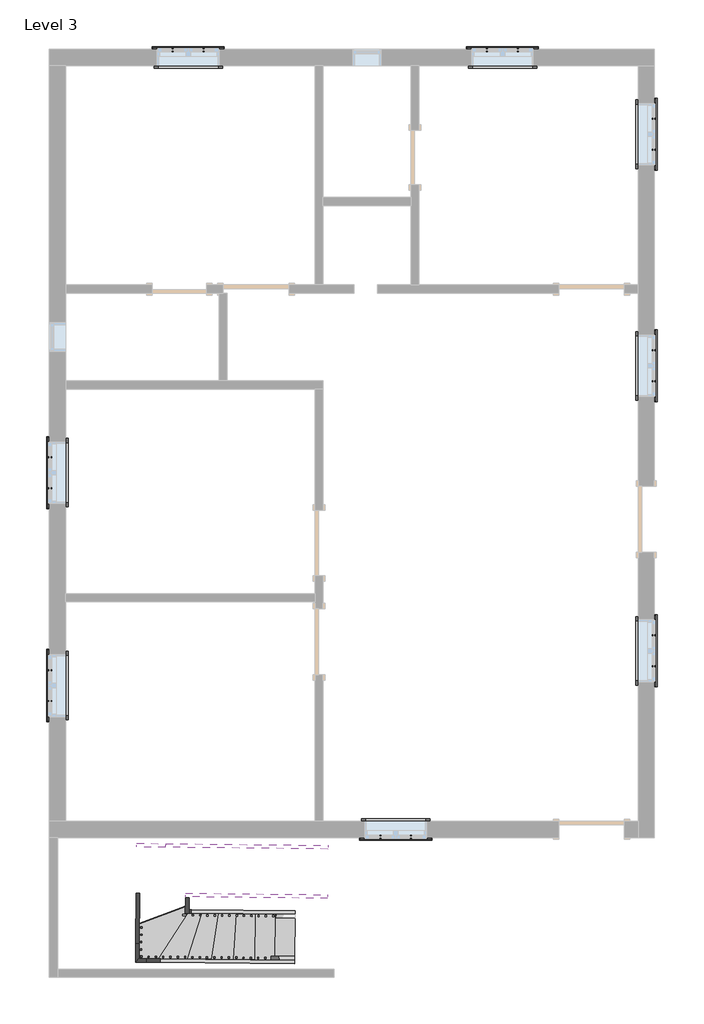
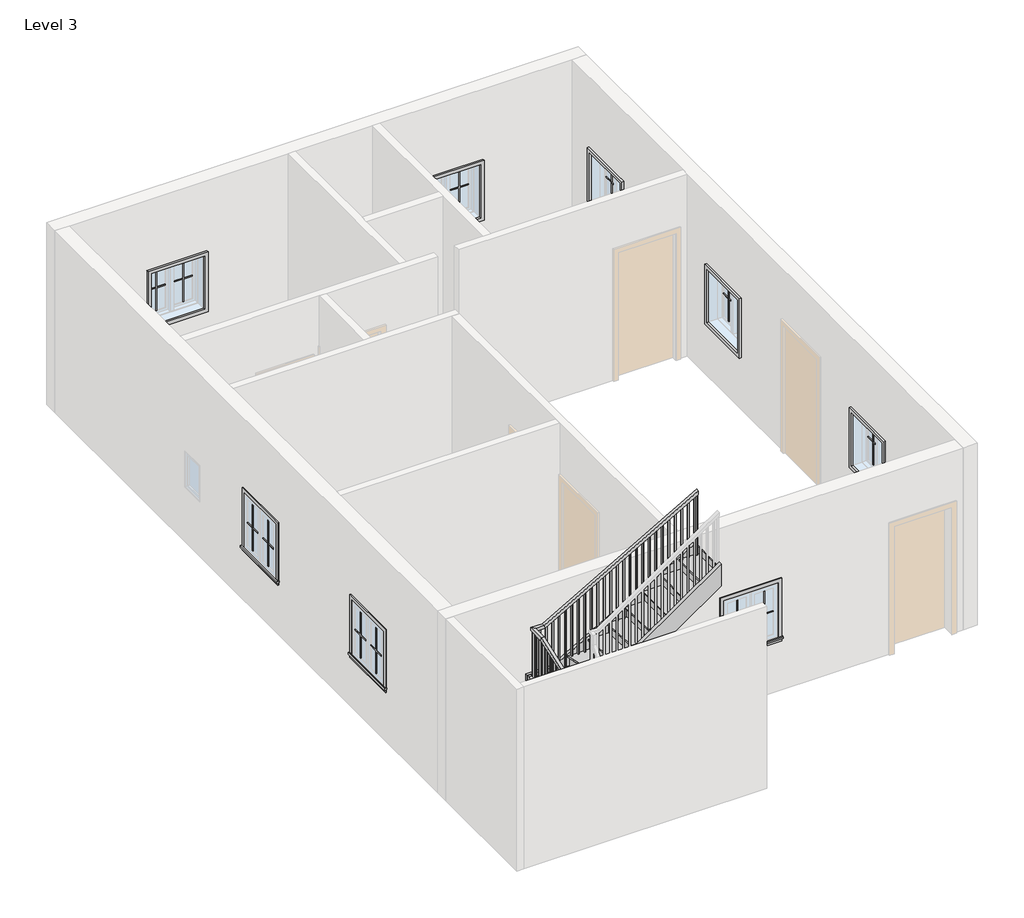
# One storey, part 2 of 2: 32 proxies, 9 members, 1 railing, 1 stair flight.
"""IFC4 building model written with IfcOpenShell, lengths in millimetres."""

from ifc_helpers import new_model, si_unit, frame, origin, place, context, project, spatial, polyline, outline, extrude, faceted_brep, transform, mapped, element, save
from components import muntin_pattern_2x2_muntin_pattern_2x2_b3fe6957, muntin_pattern_2x2_muntin_pattern_2x2_3e0ecaf2, trim_window_exterior_flat_with_sill_41619996, trim_window_interior_flat_picture_frame_51c85655, stair_flight_8b4c528d

model = new_model("IFC4")

# Units and contexts
model_context = context("Model", 3, world=origin())
ifc_project = project(units=[si_unit("LENGTHUNIT", "METRE", prefix="MILLI")], contexts=[model_context])

# Site, building, storey
site = spatial("IfcSite", under=ifc_project)
building = spatial("IfcBuilding", under=site)
storey = spatial("IfcBuildingStorey", under=building, Name="Level 3", Elevation=3200.4)

# Proxies
placement = place(None, origin())
muntin_pattern_2x2_muntin_pattern_2x2_shape = muntin_pattern_2x2_muntin_pattern_2x2_b3fe6957(model_context)
element("IfcBuildingElementProxy", 1, Name="Muntin Pattern_2x2 : Muntin Pattern_2x2", ObjectType="Muntin Pattern_2x2 : Muntin Pattern_2x2", at=placement, inside=storey, context=model_context, shape_type="MappedRepresentation", body=[
    mapped(muntin_pattern_2x2_muntin_pattern_2x2_shape, transform((-3662.5622832, 7052.6782079, 4184.65), x_axis=(1.0, 0.0, 0.0), y_axis=(0.0, 1.0, 0.0), z_axis=(0.0, 0.0, 1.0))),
])
element("IfcBuildingElementProxy", 2, Name="Muntin Pattern_2x2 : Muntin Pattern_2x2", ObjectType="Muntin Pattern_2x2 : Muntin Pattern_2x2", at=placement, inside=storey, context=model_context, shape_type="MappedRepresentation", body=[
    mapped(muntin_pattern_2x2_muntin_pattern_2x2_shape, transform((709.4127168, 7052.6782079, 4184.65), x_axis=(1.0, 0.0, 0.0), y_axis=(0.0, 1.0, 0.0), z_axis=(0.0, 0.0, 1.0))),
])
element("IfcBuildingElementProxy", 3, Name="Muntin Pattern_2x2 : Muntin Pattern_2x2", ObjectType="Muntin Pattern_2x2 : Muntin Pattern_2x2", at=placement, inside=storey, context=model_context, shape_type="MappedRepresentation", body=[
    mapped(muntin_pattern_2x2_muntin_pattern_2x2_shape, transform((3028.7502168, 6095.4157079, 4184.65), x_axis=(0.0, -1.0, 0.0), y_axis=(1.0, 0.0, 0.0), z_axis=(0.0, 0.0, 1.0))),
])
element("IfcBuildingElementProxy", 4, Name="Muntin Pattern_2x2 : Muntin Pattern_2x2", ObjectType="Muntin Pattern_2x2 : Muntin Pattern_2x2", at=placement, inside=storey, context=model_context, shape_type="MappedRepresentation", body=[
    mapped(muntin_pattern_2x2_muntin_pattern_2x2_shape, transform((3028.7502168, 2875.9657079, 4184.65), x_axis=(0.0, -1.0, 0.0), y_axis=(1.0, 0.0, 0.0), z_axis=(0.0, 0.0, 1.0))),
])
element("IfcBuildingElementProxy", 5, Name="Muntin Pattern_2x2 : Muntin Pattern_2x2", ObjectType="Muntin Pattern_2x2 : Muntin Pattern_2x2", at=placement, inside=storey, context=model_context, shape_type="MappedRepresentation", body=[
    mapped(muntin_pattern_2x2_muntin_pattern_2x2_shape, transform((3028.7502168, -1086.4342921, 4184.65), x_axis=(0.0, -1.0, 0.0), y_axis=(1.0, 0.0, 0.0), z_axis=(0.0, 0.0, 1.0))),
])
element("IfcBuildingElementProxy", 6, Name="Muntin Pattern_2x2 : Muntin Pattern_2x2", ObjectType="Muntin Pattern_2x2 : Muntin Pattern_2x2", at=placement, inside=storey, context=model_context, shape_type="MappedRepresentation", body=[
    mapped(muntin_pattern_2x2_muntin_pattern_2x2_shape, transform((-5372.2997832, 961.4407079, 4184.65), x_axis=(0.0, 1.0, 0.0), y_axis=(-1.0, 0.0, 0.0), z_axis=(0.0, 0.0, 1.0))),
])
element("IfcBuildingElementProxy", 7, Name="Muntin Pattern_2x2 : Muntin Pattern_2x2", ObjectType="Muntin Pattern_2x2 : Muntin Pattern_2x2", at=placement, inside=storey, context=model_context, shape_type="MappedRepresentation", body=[
    mapped(muntin_pattern_2x2_muntin_pattern_2x2_shape, transform((-5372.2997832, -1997.6592921, 4184.65), x_axis=(0.0, 1.0, 0.0), y_axis=(-1.0, 0.0, 0.0), z_axis=(0.0, 0.0, 1.0))),
])
element("IfcBuildingElementProxy", 8, Name="Muntin Pattern_2x2 : Muntin Pattern_2x2", ObjectType="Muntin Pattern_2x2 : Muntin Pattern_2x2", at=placement, inside=storey, context=model_context, shape_type="MappedRepresentation", body=[
    mapped(muntin_pattern_2x2_muntin_pattern_2x2_shape, transform((-347.8622832, -3888.3717921, 4184.65), x_axis=(-1.0, 0.0, 0.0), y_axis=(0.0, -1.0, 0.0), z_axis=(0.0, 0.0, 1.0))),
])
muntin_pattern_2x2_muntin_pattern_2x2_2_shape = muntin_pattern_2x2_muntin_pattern_2x2_3e0ecaf2(model_context)
element("IfcBuildingElementProxy", 9, Name="Muntin Pattern_2x2 : Muntin Pattern_2x2", ObjectType="Muntin Pattern_2x2 : Muntin Pattern_2x2", at=placement, inside=storey, context=model_context, shape_type="MappedRepresentation", body=[
    mapped(muntin_pattern_2x2_muntin_pattern_2x2_2_shape, transform((-3233.9372832, 7052.6782079, 4184.65), x_axis=(-1.0, 0.0, 0.0), y_axis=(0.0, -1.0, 0.0), z_axis=(0.0, 0.0, 1.0))),
])
element("IfcBuildingElementProxy", 10, Name="Muntin Pattern_2x2 : Muntin Pattern_2x2", ObjectType="Muntin Pattern_2x2 : Muntin Pattern_2x2", at=placement, inside=storey, context=model_context, shape_type="MappedRepresentation", body=[
    mapped(muntin_pattern_2x2_muntin_pattern_2x2_2_shape, transform((1138.0377168, 7052.6782079, 4184.65), x_axis=(-1.0, 0.0, 0.0), y_axis=(0.0, -1.0, 0.0), z_axis=(0.0, 0.0, 1.0))),
])
element("IfcBuildingElementProxy", 11, Name="Muntin Pattern_2x2 : Muntin Pattern_2x2", ObjectType="Muntin Pattern_2x2 : Muntin Pattern_2x2", at=placement, inside=storey, context=model_context, shape_type="MappedRepresentation", body=[
    mapped(muntin_pattern_2x2_muntin_pattern_2x2_2_shape, transform((3028.7502168, 5666.7907079, 4184.65), x_axis=(0.0, 1.0, 0.0), y_axis=(-1.0, 0.0, 0.0), z_axis=(0.0, 0.0, 1.0))),
])
element("IfcBuildingElementProxy", 12, Name="Muntin Pattern_2x2 : Muntin Pattern_2x2", ObjectType="Muntin Pattern_2x2 : Muntin Pattern_2x2", at=placement, inside=storey, context=model_context, shape_type="MappedRepresentation", body=[
    mapped(muntin_pattern_2x2_muntin_pattern_2x2_2_shape, transform((3028.7502168, 2447.3407079, 4184.65), x_axis=(0.0, 1.0, 0.0), y_axis=(-1.0, 0.0, 0.0), z_axis=(0.0, 0.0, 1.0))),
])
element("IfcBuildingElementProxy", 13, Name="Muntin Pattern_2x2 : Muntin Pattern_2x2", ObjectType="Muntin Pattern_2x2 : Muntin Pattern_2x2", at=placement, inside=storey, context=model_context, shape_type="MappedRepresentation", body=[
    mapped(muntin_pattern_2x2_muntin_pattern_2x2_2_shape, transform((3028.7502168, -1515.0592921, 4184.65), x_axis=(0.0, 1.0, 0.0), y_axis=(-1.0, 0.0, 0.0), z_axis=(0.0, 0.0, 1.0))),
])
element("IfcBuildingElementProxy", 14, Name="Muntin Pattern_2x2 : Muntin Pattern_2x2", ObjectType="Muntin Pattern_2x2 : Muntin Pattern_2x2", at=placement, inside=storey, context=model_context, shape_type="MappedRepresentation", body=[
    mapped(muntin_pattern_2x2_muntin_pattern_2x2_2_shape, transform((-5372.2997832, 1390.0657079, 4184.65), x_axis=(0.0, -1.0, 0.0), y_axis=(1.0, 0.0, 0.0), z_axis=(0.0, 0.0, 1.0))),
])
element("IfcBuildingElementProxy", 15, Name="Muntin Pattern_2x2 : Muntin Pattern_2x2", ObjectType="Muntin Pattern_2x2 : Muntin Pattern_2x2", at=placement, inside=storey, context=model_context, shape_type="MappedRepresentation", body=[
    mapped(muntin_pattern_2x2_muntin_pattern_2x2_2_shape, transform((-5372.2997832, -1569.0342921, 4184.65), x_axis=(0.0, -1.0, 0.0), y_axis=(1.0, 0.0, 0.0), z_axis=(0.0, 0.0, 1.0))),
])
element("IfcBuildingElementProxy", 16, Name="Muntin Pattern_2x2 : Muntin Pattern_2x2", ObjectType="Muntin Pattern_2x2 : Muntin Pattern_2x2", at=placement, inside=storey, context=model_context, shape_type="MappedRepresentation", body=[
    mapped(muntin_pattern_2x2_muntin_pattern_2x2_2_shape, transform((-776.4872832, -3888.3717921, 4184.65), x_axis=(1.0, 0.0, 0.0), y_axis=(0.0, 1.0, 0.0), z_axis=(0.0, 0.0, 1.0))),
])
trim_window_exterior_flat_with_sill_shape = trim_window_exterior_flat_with_sill_41619996(model_context)
element("IfcBuildingElementProxy", 17, Name="Trim-Window-Exterior-Flat : with Sill", ObjectType="Trim-Window-Exterior-Flat : with Sill", at=placement, inside=storey, context=model_context, shape_type="MappedRepresentation", body=[
    mapped(trim_window_exterior_flat_with_sill_shape, transform((-3448.2497832, 7062.2032079, 5029.2), x_axis=(-1.0, 0.0, 0.0), y_axis=(0.0, 0.0, 1.0), z_axis=(0.0, 1.0, 0.0))),
])
element("IfcBuildingElementProxy", 18, Name="Trim-Window-Exterior-Flat : with Sill", ObjectType="Trim-Window-Exterior-Flat : with Sill", at=placement, inside=storey, context=model_context, shape_type="MappedRepresentation", body=[
    mapped(trim_window_exterior_flat_with_sill_shape, transform((923.7252168, 7062.2032079, 5029.2), x_axis=(-1.0, 0.0, 0.0), y_axis=(0.0, 0.0, 1.0), z_axis=(0.0, 1.0, 0.0))),
])
element("IfcBuildingElementProxy", 19, Name="Trim-Window-Exterior-Flat : with Sill", ObjectType="Trim-Window-Exterior-Flat : with Sill", at=placement, inside=storey, context=model_context, shape_type="MappedRepresentation", body=[
    mapped(trim_window_exterior_flat_with_sill_shape, transform((3038.2752168, 5881.1032079, 5029.2), x_axis=(0.0, 1.0, 0.0), y_axis=(0.0, 0.0, 1.0), z_axis=(1.0, 0.0, 0.0))),
])
element("IfcBuildingElementProxy", 20, Name="Trim-Window-Exterior-Flat : with Sill", ObjectType="Trim-Window-Exterior-Flat : with Sill", at=placement, inside=storey, context=model_context, shape_type="MappedRepresentation", body=[
    mapped(trim_window_exterior_flat_with_sill_shape, transform((3038.2752168, 2661.6532079, 5029.2), x_axis=(0.0, 1.0, 0.0), y_axis=(0.0, 0.0, 1.0), z_axis=(1.0, 0.0, 0.0))),
])
element("IfcBuildingElementProxy", 21, Name="Trim-Window-Exterior-Flat : with Sill", ObjectType="Trim-Window-Exterior-Flat : with Sill", at=placement, inside=storey, context=model_context, shape_type="MappedRepresentation", body=[
    mapped(trim_window_exterior_flat_with_sill_shape, transform((3038.2752168, -1300.7467921, 5029.2), x_axis=(0.0, 1.0, 0.0), y_axis=(0.0, 0.0, 1.0), z_axis=(1.0, 0.0, 0.0))),
])
element("IfcBuildingElementProxy", 22, Name="Trim-Window-Exterior-Flat : with Sill", ObjectType="Trim-Window-Exterior-Flat : with Sill", at=placement, inside=storey, context=model_context, shape_type="MappedRepresentation", body=[
    mapped(trim_window_exterior_flat_with_sill_shape, transform((-5381.8247832, 1175.7532079, 5029.2), x_axis=(0.0, -1.0, 0.0), y_axis=(0.0, 0.0, 1.0), z_axis=(-1.0, 0.0, 0.0))),
])
element("IfcBuildingElementProxy", 23, Name="Trim-Window-Exterior-Flat : with Sill", ObjectType="Trim-Window-Exterior-Flat : with Sill", at=placement, inside=storey, context=model_context, shape_type="MappedRepresentation", body=[
    mapped(trim_window_exterior_flat_with_sill_shape, transform((-5381.8247832, -1783.3467921, 5029.2), x_axis=(0.0, -1.0, 0.0), y_axis=(0.0, 0.0, 1.0), z_axis=(-1.0, 0.0, 0.0))),
])
element("IfcBuildingElementProxy", 24, Name="Trim-Window-Exterior-Flat : with Sill", ObjectType="Trim-Window-Exterior-Flat : with Sill", at=placement, inside=storey, context=model_context, shape_type="MappedRepresentation", body=[
    mapped(trim_window_exterior_flat_with_sill_shape, transform((-562.1747832, -3897.8967921, 5029.2), x_axis=(1.0, 0.0, 0.0), y_axis=(0.0, 0.0, 1.0), z_axis=(0.0, -1.0, 0.0))),
])
trim_window_interior_flat_picture_frame_shape = trim_window_interior_flat_picture_frame_51c85655(model_context)
element("IfcBuildingElementProxy", 25, Name="Trim-Window-Interior-Flat : Picture Frame", ObjectType="Trim-Window-Interior-Flat : Picture Frame", at=placement, inside=storey, context=model_context, shape_type="MappedRepresentation", body=[
    mapped(trim_window_interior_flat_picture_frame_shape, transform((-3448.2497832, 6833.6032079, 5029.2), x_axis=(1.0, 0.0, 0.0), y_axis=(0.0, 0.0, 1.0), z_axis=(0.0, -1.0, 0.0))),
])
element("IfcBuildingElementProxy", 26, Name="Trim-Window-Interior-Flat : Picture Frame", ObjectType="Trim-Window-Interior-Flat : Picture Frame", at=placement, inside=storey, context=model_context, shape_type="MappedRepresentation", body=[
    mapped(trim_window_interior_flat_picture_frame_shape, transform((923.7252168, 6833.6032079, 5029.2), x_axis=(1.0, 0.0, 0.0), y_axis=(0.0, 0.0, 1.0), z_axis=(0.0, -1.0, 0.0))),
])
element("IfcBuildingElementProxy", 27, Name="Trim-Window-Interior-Flat : Picture Frame", ObjectType="Trim-Window-Interior-Flat : Picture Frame", at=placement, inside=storey, context=model_context, shape_type="MappedRepresentation", body=[
    mapped(trim_window_interior_flat_picture_frame_shape, transform((2809.6752168, 5881.1032079, 5029.2), x_axis=(0.0, -1.0, 0.0), y_axis=(0.0, 0.0, 1.0), z_axis=(-1.0, 0.0, 0.0))),
])
element("IfcBuildingElementProxy", 28, Name="Trim-Window-Interior-Flat : Picture Frame", ObjectType="Trim-Window-Interior-Flat : Picture Frame", at=placement, inside=storey, context=model_context, shape_type="MappedRepresentation", body=[
    mapped(trim_window_interior_flat_picture_frame_shape, transform((2809.6752168, 2661.6532079, 5029.2), x_axis=(0.0, -1.0, 0.0), y_axis=(0.0, 0.0, 1.0), z_axis=(-1.0, 0.0, 0.0))),
])
element("IfcBuildingElementProxy", 29, Name="Trim-Window-Interior-Flat : Picture Frame", ObjectType="Trim-Window-Interior-Flat : Picture Frame", at=placement, inside=storey, context=model_context, shape_type="MappedRepresentation", body=[
    mapped(trim_window_interior_flat_picture_frame_shape, transform((2809.6752168, -1300.7467921, 5029.2), x_axis=(0.0, -1.0, 0.0), y_axis=(0.0, 0.0, 1.0), z_axis=(-1.0, 0.0, 0.0))),
])
element("IfcBuildingElementProxy", 30, Name="Trim-Window-Interior-Flat : Picture Frame", ObjectType="Trim-Window-Interior-Flat : Picture Frame", at=placement, inside=storey, context=model_context, shape_type="MappedRepresentation", body=[
    mapped(trim_window_interior_flat_picture_frame_shape, transform((-5153.2247832, 1175.7532079, 5029.2), x_axis=(0.0, 1.0, 0.0), y_axis=(0.0, 0.0, 1.0), z_axis=(1.0, 0.0, 0.0))),
])
element("IfcBuildingElementProxy", 31, Name="Trim-Window-Interior-Flat : Picture Frame", ObjectType="Trim-Window-Interior-Flat : Picture Frame", at=placement, inside=storey, context=model_context, shape_type="MappedRepresentation", body=[
    mapped(trim_window_interior_flat_picture_frame_shape, transform((-5153.2247832, -1783.3467921, 5029.2), x_axis=(0.0, 1.0, 0.0), y_axis=(0.0, 0.0, 1.0), z_axis=(1.0, 0.0, 0.0))),
])
element("IfcBuildingElementProxy", 32, Name="Trim-Window-Interior-Flat : Picture Frame", ObjectType="Trim-Window-Interior-Flat : Picture Frame", at=placement, inside=storey, context=model_context, shape_type="MappedRepresentation", body=[
    mapped(trim_window_interior_flat_picture_frame_shape, transform((-562.1747832, -3669.2967921, 5029.2), x_axis=(-1.0, 0.0, 0.0), y_axis=(0.0, 0.0, 1.0), z_axis=(0.0, 1.0, 0.0))),
])

# Members
element("IfcMember", 33, ObjectType="Stringer - 2\" Width", at=placement, inside=storey, context=model_context, shape_type="SweptSolid", body=[
    extrude(outline(polyline([(-105.6395382, -202.4353776), (0.0, 0.0), (2328.2458671, 0.0), (2169.1880402, -304.8), (90.52017, -304.8), (-105.6395382, -202.4353776)])), frame((-1968.9977307, -5651.1672049, 3428.7413982), z_axis=(0.01073603161956522, 0.9999423671517593, 0.0), x_axis=(-0.8864958884204133, 0.009517996437940358, 0.4626385711951714)), (0.0, 0.0, 1.0), 50.8),
])
element("IfcMember", 34, ObjectType="Stringer - 2\" Width", at=placement, inside=storey, context=model_context, shape_type="SweptSolid", body=[
    extrude(outline(polyline([(-4032.4327287, -5578.2098967), (-4032.9781191, -5629.006969), (-4182.4018504, -5627.4026586), (-4131.0593878, -5577.1509768), (-4032.4327287, -5578.2098967)])), frame((0.0, 0.0, 4162.0719334), z_axis=(0.0, 0.0, 1.0), x_axis=(1.0, 0.0, 0.0)), (0.0, 0.0, 1.0), 343.8058061),
])
element("IfcMember", 35, ObjectType="Stringer - 2\" Width", at=placement, inside=storey, context=model_context, shape_type="SweptSolid", body=[
    extrude(outline(polyline([(-4131.0593878, -5577.1509768), (-4182.4018504, -5627.4026586), (-4179.6442274, -5370.5606366), (-4128.8471552, -5371.106027), (-4131.0593878, -5577.1509768)])), frame((0.0, 0.0, 4162.0719334), z_axis=(0.0, 0.0, 1.0), x_axis=(1.0, 0.0, 0.0)), (0.0, 0.0, 1.0), 343.8058061),
])
element("IfcMember", 36, ObjectType="Stringer - 2\" Width", at=placement, inside=storey, context=model_context, shape_type="SweptSolid", body=[
    extrude(outline(polyline([(110.9788635, -325.4014815), (0.0, 0.0), (1419.3210826, 0.0), (1526.5904374, -314.5248191), (1494.6989405, -325.4014816), (110.9788635, -325.4014815)])), frame((-4128.8471552, -5371.106027, 4162.0719334), z_axis=(-0.9999423671517593, 0.010736031619565316, 0.0), x_axis=(0.010161319362697884, 0.946414289466532, 0.3227951986668462)), (0.0, 0.0, 1.0), 50.8),
])
element("IfcMember", 37, ObjectType="Stringer - 2\" Width", at=placement, inside=storey, context=model_context, shape_type="SweptSolid", body=[
    extrude(outline(polyline([(-4165.2220526, -4027.2948827), (-4164.6766622, -3976.4978105), (-3763.6581151, -3980.8034064), (-3764.2035055, -4031.6004787), (-4165.2220526, -4027.2948827)])), frame((0.0, 0.0, 4630.4968076), z_axis=(0.0, 0.0, 1.0), x_axis=(1.0, 0.0, 0.0)), (0.0, 0.0, 1.0), 322.0391291),
])
element("IfcMember", 38, ObjectType="Stringer - 2\" Width", at=placement, inside=storey, context=model_context, shape_type="SweptSolid", body=[
    extrude(outline(polyline([(-111.9640108, -160.4153284), (0.0, 0.0), (1801.1015507, 0.0), (1588.362339, -304.8), (94.9016984, -304.8), (-111.9640108, -160.4153284)])), frame((-1961.6349602, -4965.4067295, 3396.0246848), z_axis=(0.010736031619565368, 0.9999423671517593, 0.0), x_axis=(-0.8199685195580251, 0.008803715336213087, 0.5723409137307062)), (0.0, 0.0, 1.0), 50.8),
])
element("IfcMember", 39, ObjectType="Stringer - 2\" Width", at=placement, inside=storey, context=model_context, shape_type="SweptSolid", body=[
    extrude(outline(polyline([(451.3522078, -304.8), (7.554265, -5.1014262), (10.999279, 0.0), (408.4725128, 0.0), (831.8908901, -285.9361695), (819.1520678, -304.8), (451.3522078, -304.8)])), frame((-3438.4815323, -4949.5503441, 4081.5097108), z_axis=(-0.9999423671517593, 0.010736031619565902, 0.0), x_axis=(0.006008376943933788, 0.559613726649971, 0.8287317879455518)), (0.0, 0.0, 1.0), 50.8),
])
element("IfcMember", 40, ObjectType="Stringer - 2\" Width", at=placement, inside=storey, context=model_context, shape_type="SweptSolid", body=[
    extrude(outline(polyline([(215.732707, -304.8), (0.0, 0.0), (2421.4097535, 0.0), (2637.1424605, -304.8), (215.732707, -304.8)])), frame((-3486.8243477, -4720.4181286, 4557.5256311), z_axis=(0.010736031619565212, 0.9999423671517593, 0.0), x_axis=(0.8161886957592968, -0.008763132689499907, 0.5777189804915572)), (0.0, 0.0, 1.0), 50.8),
])
element("IfcMember", 41, ObjectType="Stringer - 2\" Width", at=placement, inside=storey, context=model_context, shape_type="SweptSolid", body=[
    extrude(outline(polyline([(161.6856691, -278.5084291), (0.0, 0.0), (2614.6236412, 0.0), (2776.3093103, -278.508429), (161.6856691, -278.5084291)])), frame((-3764.2035055, -4031.6004787, 4630.4968076), z_axis=(0.010736031619565317, 0.9999423671517593, 0.0), x_axis=(0.8647780740833303, -0.009284819857879245, 0.5020683964410952)), (0.0, 0.0, 1.0), 50.8),
])

# Railing
element("IfcRailing", 42, ObjectType="Handrail - Rectangular", at=placement, inside=storey, context=model_context, shape_type="SolidModel", body=[
    faceted_brep([(-1968.4523403, -5600.3701326, 4284.1333333), (-1968.4523403, -5600.3701326, 4226.5388957), (-1967.9069499, -5549.5730604, 4226.5388957), (-1967.9069499, -5549.5730604, 4284.1333333), (-4009.5042766, -5578.4560715, 5374.5579081), (-4022.2220752, -5578.319525, 5323.7579081), (-4021.6766848, -5527.5224527, 5323.7579081), (-4008.9588862, -5527.6589993, 5374.5579081), (-4131.0593878, -5577.1509768, 5374.5579081), (-4131.0593878, -5577.1509768, 5323.7579081), (-4079.7169251, -5526.8992949, 5323.7579081), (-4079.7169251, -5526.8992949, 5374.5579081), (-4129.1695675, -5401.1351667, 5374.5579081), (-4129.079122, -5392.7111679, 5323.7579081), (-4078.2820498, -5393.2565584, 5323.7579081), (-4078.3724953, -5401.6805571, 5374.5579081), (-4117.5603361, -4319.8639155, 5743.3490097), (-4117.4698906, -4311.4399167, 5692.5490097), (-4066.6728183, -4311.9853071, 5692.5490097), (-4066.7632639, -4320.4093059, 5743.3490097), (-4114.4249804, -4027.8402731, 5743.3490097), (-4114.4249804, -4027.8402731, 5692.5490097), (-4064.1732985, -4079.1827358, 5692.5490097), (-4064.1732985, -4079.1827358, 5743.3490097), (-3933.3337165, -4029.7845867, 5743.3490097), (-3919.5861077, -4029.93219, 5692.5490097), (-3920.1314981, -4080.7292622, 5692.5490097), (-3933.8791069, -4080.581659, 5743.3490097), (-1503.1343086, -4055.8767882, 7162.8), (-1503.679699, -4106.6738604, 7162.8), (-1503.679699, -4106.6738604, 7103.9701828), (-1503.1343086, -4055.8767882, 7103.9701828)], [[[0, 1, 2, 3]], [[1, 0, 4, 5]], [[2, 1, 5, 6]], [[3, 2, 6, 7]], [[0, 3, 7, 4]], [[5, 4, 8, 9]], [[6, 5, 9, 10]], [[7, 6, 10, 11]], [[4, 7, 11, 8]], [[9, 8, 12, 13]], [[10, 9, 13, 14]], [[11, 10, 14, 15]], [[8, 11, 15, 12]], [[13, 12, 16, 17]], [[14, 13, 17, 18]], [[15, 14, 18, 19]], [[12, 15, 19, 16]], [[17, 16, 20, 21]], [[18, 17, 21, 22]], [[19, 18, 22, 23]], [[16, 19, 23, 20]], [[21, 20, 24, 25]], [[22, 21, 25, 26]], [[23, 22, 26, 27]], [[20, 23, 27, 24]], [[28, 29, 30, 31]], [[25, 24, 28, 31]], [[26, 25, 31, 30]], [[27, 26, 30, 29]], [[24, 27, 29, 28]]]),
    extrude(outline(polyline([(234.1631202, 19.05), (1226.6129544, 19.05), (1226.6129544, 0.0), (223.0368797, 0.0), (234.1631202, 19.05)])), frame((-1540.0233365, -4090.4077365, 7305.6796211), z_axis=(0.010736031619565153, 0.9999423671517594, 0.0), x_axis=(0.0, 0.0, -1.0)), (0.0, 0.0, 1.0), 19.05),
    extrude(outline(polyline([(234.1631202, 19.05), (1167.2730054, 19.05), (1167.2730054, 0.0), (223.0368798, 0.0), (234.1631202, 19.05)])), frame((-1641.617481, -4089.3169557, 7246.3396721), z_axis=(0.010736031619565153, 0.9999423671517594, 0.0), x_axis=(0.0, 0.0, -1.0)), (0.0, 0.0, 1.0), 19.05),
    extrude(outline(polyline([(234.1631202, 19.05), (1107.9330563, 19.05), (1107.9330563, 0.0), (223.0368797, 0.0), (234.1631202, 19.05)])), frame((-1743.2116255, -4088.2261749, 7186.999723), z_axis=(0.010736031619565153, 0.9999423671517594, 0.0), x_axis=(0.0, 0.0, -1.0)), (0.0, 0.0, 1.0), 19.05),
    extrude(outline(polyline([(234.1631202, 19.05), (1217.9264407, 19.05), (1217.9264407, 0.0), (223.0368798, 0.0), (234.1631202, 19.05)])), frame((-1844.80577, -4087.1353941, 7127.659774), z_axis=(0.010736031619565153, 0.9999423671517594, 0.0), x_axis=(0.0, 0.0, -1.0)), (0.0, 0.0, 1.0), 19.05),
    extrude(outline(polyline([(234.1631203, 19.05), (1158.5864917, 19.05), (1158.5864917, 0.0), (223.0368798, 0.0), (234.1631203, 19.05)])), frame((-1946.3999145, -4086.0446133, 7068.319825), z_axis=(0.010736031619565153, 0.9999423671517594, 0.0), x_axis=(0.0, 0.0, -1.0)), (0.0, 0.0, 1.0), 19.05),
    extrude(outline(polyline([(234.1631202, 19.05), (1099.2465426, 19.05), (1099.2465426, 0.0), (223.0368798, 0.0), (234.1631202, 19.05)])), frame((-2047.994059, -4084.9538324, 7008.9798759), z_axis=(0.010736031619565153, 0.9999423671517594, 0.0), x_axis=(0.0, 0.0, -1.0)), (0.0, 0.0, 1.0), 19.05),
    extrude(outline(polyline([(234.1631202, 19.0499999), (1209.2399269, 19.0499999), (1209.2399269, 0.0), (223.0368798, 0.0), (234.1631202, 19.0499999)])), frame((-2149.5882036, -4083.8630516, 6949.6399269), z_axis=(0.010736031619565153, 0.9999423671517594, 0.0), x_axis=(0.0, 0.0, -1.0)), (0.0, 0.0, 1.0), 19.05),
    extrude(outline(polyline([(234.1631202, 19.0499999), (1149.8999778, 19.0499999), (1149.8999778, 0.0), (223.0368797, 0.0), (234.1631202, 19.0499999)])), frame((-2251.1823481, -4082.7722708, 6890.2999778), z_axis=(0.010736031619565153, 0.9999423671517594, 0.0), x_axis=(0.0, 0.0, -1.0)), (0.0, 0.0, 1.0), 19.05),
    extrude(outline(polyline([(234.1631202, 19.05), (1259.8933621, 19.05), (1259.8933621, 0.0), (223.0368798, 0.0), (234.1631202, 19.05)])), frame((-2352.7764926, -4081.68149, 6830.9600288), z_axis=(0.010736031619565153, 0.9999423671517594, 0.0), x_axis=(0.0, 0.0, -1.0)), (0.0, 0.0, 1.0), 19.05),
    extrude(outline(polyline([(234.1631203, 19.05), (1200.5534131, 19.05), (1200.5534131, 0.0), (223.0368798, 0.0), (234.1631203, 19.05)])), frame((-2454.3706371, -4080.5907092, 6771.6200798), z_axis=(0.010736031619565153, 0.9999423671517594, 0.0), x_axis=(0.0, 0.0, -1.0)), (0.0, 0.0, 1.0), 19.05),
    extrude(outline(polyline([(234.1631202, 19.05), (1141.213464, 19.05), (1141.213464, 0.0), (223.0368798, 0.0), (234.1631202, 19.05)])), frame((-2555.9647816, -4079.4999284, 6712.2801307), z_axis=(0.010736031619565153, 0.9999423671517594, 0.0), x_axis=(0.0, 0.0, -1.0)), (0.0, 0.0, 1.0), 19.05),
    extrude(outline(polyline([(234.1631203, 19.05), (1251.2068484, 19.05), (1251.2068484, 0.0), (223.0368798, 0.0), (234.1631203, 19.05)])), frame((-2657.5589261, -4078.4091476, 6652.9401817), z_axis=(0.010736031619565153, 0.9999423671517594, 0.0), x_axis=(0.0, 0.0, -1.0)), (0.0, 0.0, 1.0), 19.05),
    extrude(outline(polyline([(234.1631202, 19.05), (1191.8668993, 19.05), (1191.8668993, 0.0), (223.0368797, 0.0), (234.1631202, 19.05)])), frame((-2759.1530706, -4077.3183668, 6593.6002326), z_axis=(0.010736031619565153, 0.9999423671517594, 0.0), x_axis=(0.0, 0.0, -1.0)), (0.0, 0.0, 1.0), 19.05),
    extrude(outline(polyline([(234.1631202, 19.05), (1132.5269503, 19.05), (1132.5269503, 0.0), (223.0368798, 0.0), (234.1631202, 19.05)])), frame((-2860.7472151, -4076.2275859, 6534.2602836), z_axis=(0.010736031619565153, 0.9999423671517594, 0.0), x_axis=(0.0, 0.0, -1.0)), (0.0, 0.0, 1.0), 19.05),
    extrude(outline(polyline([(234.1631202, 19.05), (1242.5203345, 19.05), (1242.5203345, 0.0), (223.0368797, 0.0), (234.1631202, 19.05)])), frame((-2962.3413596, -4075.1368051, 6474.9203345), z_axis=(0.010736031619565153, 0.9999423671517594, 0.0), x_axis=(0.0, 0.0, -1.0)), (0.0, 0.0, 1.0), 19.05),
    extrude(outline(polyline([(234.1631202, 19.05), (1183.1803855, 19.05), (1183.1803855, 0.0), (223.0368798, 0.0), (234.1631202, 19.05)])), frame((-3063.9355041, -4074.0460243, 6415.5803855), z_axis=(0.010736031619565153, 0.9999423671517594, 0.0), x_axis=(0.0, 0.0, -1.0)), (0.0, 0.0, 1.0), 19.05),
    extrude(outline(polyline([(234.1631203, 19.05), (1123.8404365, 19.05), (1123.8404365, 0.0), (223.0368798, 0.0), (234.1631203, 19.05)])), frame((-3165.5296486, -4072.9552435, 6356.2404365), z_axis=(0.010736031619565153, 0.9999423671517594, 0.0), x_axis=(0.0, 0.0, -1.0)), (0.0, 0.0, 1.0), 19.05),
    extrude(outline(polyline([(234.1631202, 19.05), (1233.8338207, 19.05), (1233.8338207, 0.0), (223.0368798, 0.0), (234.1631202, 19.05)])), frame((-3267.1237931, -4071.8644627, 6296.9004874), z_axis=(0.010736031619565153, 0.9999423671517594, 0.0), x_axis=(0.0, 0.0, -1.0)), (0.0, 0.0, 1.0), 19.05),
    extrude(outline(polyline([(234.1631202, 19.05), (1174.4938717, 19.05), (1174.4938717, 0.0), (223.0368798, 0.0), (234.1631202, 19.05)])), frame((-3368.7179376, -4070.7736819, 6237.5605384), z_axis=(0.010736031619565153, 0.9999423671517594, 0.0), x_axis=(0.0, 0.0, -1.0)), (0.0, 0.0, 1.0), 19.05),
    extrude(outline(polyline([(234.1631202, 19.05), (1115.1539226, 19.05), (1115.1539226, 0.0), (223.0368797, 0.0), (234.1631202, 19.05)])), frame((-3470.3120821, -4069.6829011, 6178.2205893), z_axis=(0.010736031619565153, 0.9999423671517594, 0.0), x_axis=(0.0, 0.0, -1.0)), (0.0, 0.0, 1.0), 19.05),
    extrude(outline(polyline([(234.1631202, 19.05), (1225.147307, 19.05), (1225.147307, 0.0), (223.0368798, 0.0), (234.1631202, 19.05)])), frame((-3571.9062266, -4068.5921203, 6118.8806403), z_axis=(0.010736031619565153, 0.9999423671517594, 0.0), x_axis=(0.0, 0.0, -1.0)), (0.0, 0.0, 1.0), 19.05),
    extrude(outline(polyline([(234.1631202, 19.05), (1165.8073579, 19.05), (1165.8073579, 0.0), (223.0368797, 0.0), (234.1631202, 19.05)])), frame((-3673.5003711, -4067.5013394, 6059.5406912), z_axis=(0.010736031619565153, 0.9999423671517594, 0.0), x_axis=(0.0, 0.0, -1.0)), (0.0, 0.0, 1.0), 19.05),
    extrude(outline(polyline([(234.1631202, 19.05), (1106.4674089, 19.05), (1106.4674089, 0.0), (223.0368798, 0.0), (234.1631202, 19.05)])), frame((-3775.0945156, -4066.4105586, 6000.2007422), z_axis=(0.010736031619565153, 0.9999423671517594, 0.0), x_axis=(0.0, 0.0, -1.0)), (0.0, 0.0, 1.0), 19.05),
    extrude(outline(polyline([(234.1631203, 19.05), (1047.1274599, 19.05), (1047.1274599, 0.0), (223.0368798, 0.0), (234.1631203, 19.05)])), frame((-3876.6886601, -4065.3197778, 5940.8607932), z_axis=(0.010736031619565153, 0.9999423671517594, 0.0), x_axis=(0.0, 0.0, -1.0)), (0.0, 0.0, 1.0), 19.05),
    extrude(outline(polyline([(-3997.1271853, -4044.9755735), (-3978.0782832, -4045.1800949), (-3978.2828046, -4064.228997), (-3997.3317067, -4064.0244756), (-3997.1271853, -4044.9755735)])), frame((0.0, 0.0, 4893.7333333), z_axis=(0.0, 0.0, 1.0), x_axis=(1.0, 0.0, 0.0)), (0.0, 0.0, 1.0), 798.8156763),
    extrude(outline(polyline([(-4099.7439368, -4139.1293032), (-4099.5394154, -4120.0804011), (-4080.4905133, -4120.2849225), (-4080.6950347, -4139.3338246), (-4099.7439368, -4139.1293032)])), frame((0.0, 0.0, 4893.7333333), z_axis=(0.0, 0.0, 1.0), x_axis=(1.0, 0.0, 0.0)), (0.0, 0.0, 1.0), 798.8156763),
    extrude(outline(polyline([(-4100.8347176, -4240.7234477), (-4100.6301962, -4221.6745456), (-4081.5812941, -4221.879067), (-4081.7858155, -4240.9279691), (-4100.8347176, -4240.7234477)])), frame((0.0, 0.0, 4724.4), z_axis=(0.0, 0.0, 1.0), x_axis=(1.0, 0.0, 0.0)), (0.0, 0.0, 1.0), 968.1490097),
    extrude(outline(polyline([(231.8485214, 19.05), (1189.524158, 19.05), (1189.524158, 0.0), (225.3514786, 0.0), (231.8485214, 19.05)])), frame((-4082.6720749, -4323.4732115, 5913.924158), z_axis=(-0.9999423671517593, 0.010736031619565137, 0.0), x_axis=(0.0, 0.0, -1.0)), (0.0, 0.0, 1.0), 19.05),
    extrude(outline(polyline([(231.8485214, 19.05), (1154.8732631, 19.05), (1154.8732631, 0.0), (225.3514786, 0.0), (231.8485214, 19.05)])), frame((-4083.7628557, -4425.067356, 5879.2732631), z_axis=(-0.9999423671517593, 0.010736031619565137, 0.0), x_axis=(0.0, 0.0, -1.0)), (0.0, 0.0, 1.0), 19.05),
    extrude(outline(polyline([(231.8485214, 19.05), (1120.2223682, 19.05), (1120.2223682, 0.0), (225.3514786, 0.0), (231.8485214, 19.05)])), frame((-4084.8536366, -4526.6615005, 5844.6223682), z_axis=(-0.9999423671517593, 0.010736031619565137, 0.0), x_axis=(0.0, 0.0, -1.0)), (0.0, 0.0, 1.0), 19.05),
    extrude(outline(polyline([(231.8485214, 19.05), (1085.5714733, 19.05), (1085.5714733, 0.0), (225.3514786, 0.0), (231.8485214, 19.05)])), frame((-4085.9444174, -4628.255645, 5809.9714733), z_axis=(-0.9999423671517593, 0.010736031619565137, 0.0), x_axis=(0.0, 0.0, -1.0)), (0.0, 0.0, 1.0), 19.05),
    extrude(outline(polyline([(231.8485214, 19.05), (1220.2539118, 19.05), (1220.2539118, 0.0), (225.3514786, 0.0), (231.8485214, 19.05)])), frame((-4087.0351982, -4729.8497895, 5775.3205785), z_axis=(-0.9999423671517593, 0.010736031619565137, 0.0), x_axis=(0.0, 0.0, -1.0)), (0.0, 0.0, 1.0), 19.05),
    extrude(outline(polyline([(231.8485214, 19.05), (1185.6030169, 19.05), (1185.6030169, 0.0), (225.3514786, 0.0), (231.8485214, 19.05)])), frame((-4088.125979, -4831.443934, 5740.6696836), z_axis=(-0.9999423671517593, 0.010736031619565137, 0.0), x_axis=(0.0, 0.0, -1.0)), (0.0, 0.0, 1.0), 19.05),
    extrude(outline(polyline([(231.8485214, 19.05), (1150.952122, 19.05), (1150.952122, 0.0), (225.3514786, 0.0), (231.8485214, 19.05)])), frame((-4089.2167598, -4933.0380785, 5706.0187887), z_axis=(-0.9999423671517593, 0.010736031619565137, 0.0), x_axis=(0.0, 0.0, -1.0)), (0.0, 0.0, 1.0), 19.05),
    extrude(outline(polyline([(231.8485214, 19.05), (1116.3012271, 19.05), (1116.3012271, 0.0), (225.3514786, 0.0), (231.8485214, 19.05)])), frame((-4090.3075406, -5034.632223, 5671.3678938), z_axis=(-0.9999423671517593, 0.010736031619565137, 0.0), x_axis=(0.0, 0.0, -1.0)), (0.0, 0.0, 1.0), 19.05),
    extrude(outline(polyline([(231.8485214, 19.05), (1250.9836656, 19.05), (1250.9836656, 0.0), (225.3514786, 0.0), (231.8485214, 19.05)])), frame((-4091.3983214, -5136.2263675, 5636.7169989), z_axis=(-0.9999423671517593, 0.010736031619565137, 0.0), x_axis=(0.0, 0.0, -1.0)), (0.0, 0.0, 1.0), 19.05),
    extrude(outline(polyline([(231.8485214, 19.05), (1216.3327708, 19.05), (1216.3327708, 0.0), (225.3514786, 0.0), (231.8485214, 19.05)])), frame((-4092.4891022, -5237.820512, 5602.0661041), z_axis=(-0.9999423671517593, 0.010736031619565137, 0.0), x_axis=(0.0, 0.0, -1.0)), (0.0, 0.0, 1.0), 19.05),
    extrude(outline(polyline([(231.8485214, 19.05), (1181.6818759, 19.05), (1181.6818759, 0.0), (225.3514786, 0.0), (231.8485214, 19.05)])), frame((-4093.5798831, -5339.4146565, 5567.4152092), z_axis=(-0.9999423671517593, 0.010736031619565137, 0.0), x_axis=(0.0, 0.0, -1.0)), (0.0, 0.0, 1.0), 19.05),
    extrude(outline(polyline([(-4113.9240874, -5459.8531817), (-4113.719566, -5440.8042796), (-4094.6706639, -5441.008801), (-4094.8751853, -5460.0577031), (-4113.9240874, -5459.8531817)])), frame((0.0, 0.0, 4385.7333333), z_axis=(0.0, 0.0, 1.0), x_axis=(1.0, 0.0, 0.0)), (0.0, 0.0, 1.0), 938.0245748),
    extrude(outline(polyline([(-4092.2344893, -5561.6919112), (-4111.2833914, -5561.4873898), (-4111.07887, -5542.4384877), (-4092.0299679, -5542.6430091), (-4092.2344893, -5561.6919112)])), frame((0.0, 0.0, 4385.7333333), z_axis=(0.0, 0.0, 1.0), x_axis=(1.0, 0.0, 0.0)), (0.0, 0.0, 1.0), 938.0245748),
    extrude(outline(polyline([(223.5115966, 19.05), (1154.9316075, 19.05), (1154.9316075, 0.0), (233.6884033, 0.0), (223.5115966, 19.05)])), frame((-3990.6403448, -5562.782692, 5540.6649408), z_axis=(0.010736031619565252, 0.9999423671517594, 0.0), x_axis=(0.0, 0.0, -1.0)), (0.0, 0.0, 1.0), 19.05),
    extrude(outline(polyline([(223.5115967, 19.05), (1100.6553053, 19.05), (1100.6553053, 0.0), (233.6884034, 0.0), (223.5115967, 19.05)])), frame((-3889.0462003, -5563.8734728, 5486.3886386), z_axis=(0.010736031619565252, 0.9999423671517594, 0.0), x_axis=(0.0, 0.0, -1.0)), (0.0, 0.0, 1.0), 19.05),
    extrude(outline(polyline([(223.5115967, 19.05), (1215.7123363, 19.05), (1215.7123363, 0.0), (233.6884033, 0.0), (223.5115967, 19.05)])), frame((-3787.4520558, -5564.9642536, 5432.1123363), z_axis=(0.010736031619565252, 0.9999423671517594, 0.0), x_axis=(0.0, 0.0, -1.0)), (0.0, 0.0, 1.0), 19.05),
    extrude(outline(polyline([(223.5115967, 19.05), (1161.4360341, 19.05), (1161.4360341, 0.0), (233.6884034, 0.0), (223.5115967, 19.05)])), frame((-3685.8579113, -5566.0550344, 5377.8360341), z_axis=(0.010736031619565252, 0.9999423671517594, 0.0), x_axis=(0.0, 0.0, -1.0)), (0.0, 0.0, 1.0), 19.05),
    extrude(outline(polyline([(223.5115967, 19.05), (1107.1597318, 19.05), (1107.1597318, 0.0), (233.6884033, 0.0), (223.5115967, 19.05)])), frame((-3584.2637668, -5567.1458152, 5323.5597318), z_axis=(0.010736031619565252, 0.9999423671517594, 0.0), x_axis=(0.0, 0.0, -1.0)), (0.0, 0.0, 1.0), 19.05),
    extrude(outline(polyline([(223.5115966, 19.05), (1052.8834295, 19.05), (1052.8834295, 0.0), (233.6884033, 0.0), (223.5115966, 19.05)])), frame((-3482.6696223, -5568.236596, 5269.2834295), z_axis=(0.010736031619565252, 0.9999423671517594, 0.0), x_axis=(0.0, 0.0, -1.0)), (0.0, 0.0, 1.0), 19.05),
    extrude(outline(polyline([(223.5115967, 19.05), (1167.9404606, 19.05), (1167.9404606, 0.0), (233.6884034, 0.0), (223.5115967, 19.05)])), frame((-3381.0754778, -5569.3273769, 5215.0071273), z_axis=(0.010736031619565252, 0.9999423671517594, 0.0), x_axis=(0.0, 0.0, -1.0)), (0.0, 0.0, 1.0), 19.05),
    extrude(outline(polyline([(223.5115966, 19.05), (1113.6641583, 19.05), (1113.6641583, 0.0), (233.6884033, 0.0), (223.5115966, 19.05)])), frame((-3279.4813333, -5570.4181577, 5160.730825), z_axis=(0.010736031619565252, 0.9999423671517594, 0.0), x_axis=(0.0, 0.0, -1.0)), (0.0, 0.0, 1.0), 19.05),
    extrude(outline(polyline([(223.5115967, 19.05), (1059.3878561, 19.05), (1059.3878561, 0.0), (233.6884034, 0.0), (223.5115967, 19.05)])), frame((-3177.8871888, -5571.5089385, 5106.4545228), z_axis=(0.010736031619565252, 0.9999423671517594, 0.0), x_axis=(0.0, 0.0, -1.0)), (0.0, 0.0, 1.0), 19.05),
    extrude(outline(polyline([(223.5115966, 19.05), (1174.4448872, 19.05), (1174.4448872, 0.0), (233.6884033, 0.0), (223.5115966, 19.05)])), frame((-3076.2930443, -5572.5997193, 5052.1782205), z_axis=(0.010736031619565252, 0.9999423671517594, 0.0), x_axis=(0.0, 0.0, -1.0)), (0.0, 0.0, 1.0), 19.05),
    extrude(outline(polyline([(223.5115967, 19.05), (1120.168585, 19.05), (1120.168585, 0.0), (233.6884034, 0.0), (223.5115967, 19.05)])), frame((-2974.6988998, -5573.6905001, 4997.9019183), z_axis=(0.010736031619565252, 0.9999423671517594, 0.0), x_axis=(0.0, 0.0, -1.0)), (0.0, 0.0, 1.0), 19.05),
    extrude(outline(polyline([(223.5115967, 19.05), (1065.8922827, 19.05), (1065.8922827, 0.0), (233.6884033, 0.0), (223.5115967, 19.05)])), frame((-2873.1047553, -5574.7812809, 4943.625616), z_axis=(0.010736031619565252, 0.9999423671517594, 0.0), x_axis=(0.0, 0.0, -1.0)), (0.0, 0.0, 1.0), 19.05),
    extrude(outline(polyline([(223.5115966, 19.05), (1180.9493137, 19.05), (1180.9493137, 0.0), (233.6884033, 0.0), (223.5115966, 19.05)])), frame((-2771.5106108, -5575.8720617, 4889.3493137), z_axis=(0.010736031619565252, 0.9999423671517594, 0.0), x_axis=(0.0, 0.0, -1.0)), (0.0, 0.0, 1.0), 19.05),
    extrude(outline(polyline([(223.5115967, 19.05), (1126.6730115, 19.05), (1126.6730115, 0.0), (233.6884033, 0.0), (223.5115967, 19.05)])), frame((-2669.9164663, -5576.9628425, 4835.0730115), z_axis=(0.010736031619565252, 0.9999423671517594, 0.0), x_axis=(0.0, 0.0, -1.0)), (0.0, 0.0, 1.0), 19.05),
    extrude(outline(polyline([(223.5115966, 19.0499999), (1072.3967092, 19.0499999), (1072.3967092, 0.0), (233.6884033, 0.0), (223.5115966, 19.0499999)])), frame((-2568.3223218, -5578.0536234, 4780.7967092), z_axis=(0.010736031619565252, 0.9999423671517594, 0.0), x_axis=(0.0, 0.0, -1.0)), (0.0, 0.0, 1.0), 19.05),
    extrude(outline(polyline([(223.5115967, 19.0499999), (1187.4537403, 19.0499999), (1187.4537403, 0.0), (233.6884034, 0.0), (223.5115967, 19.0499999)])), frame((-2466.7281773, -5579.1444042, 4726.520407), z_axis=(0.010736031619565252, 0.9999423671517594, 0.0), x_axis=(0.0, 0.0, -1.0)), (0.0, 0.0, 1.0), 19.05),
    extrude(outline(polyline([(223.5115966, 19.05), (1133.177438, 19.05), (1133.177438, 0.0), (233.6884033, 0.0), (223.5115966, 19.05)])), frame((-2365.1340327, -5580.235185, 4672.2441047), z_axis=(0.010736031619565252, 0.9999423671517594, 0.0), x_axis=(0.0, 0.0, -1.0)), (0.0, 0.0, 1.0), 19.05),
    extrude(outline(polyline([(223.5115967, 19.05), (1078.9011358, 19.05), (1078.9011358, 0.0), (233.6884034, 0.0), (223.5115967, 19.05)])), frame((-2263.5398882, -5581.3259658, 4617.9678025), z_axis=(0.010736031619565252, 0.9999423671517594, 0.0), x_axis=(0.0, 0.0, -1.0)), (0.0, 0.0, 1.0), 19.05),
    extrude(outline(polyline([(223.5115967, 19.05), (1193.9581669, 19.05), (1193.9581669, 0.0), (233.6884033, 0.0), (223.5115967, 19.05)])), frame((-2161.9457437, -5582.4167466, 4563.6915002), z_axis=(0.010736031619565252, 0.9999423671517594, 0.0), x_axis=(0.0, 0.0, -1.0)), (0.0, 0.0, 1.0), 19.05),
    extrude(outline(polyline([(223.5115967, 19.05), (1139.6818647, 19.05), (1139.6818647, 0.0), (233.6884034, 0.0), (223.5115967, 19.05)])), frame((-2060.3515992, -5583.5075274, 4509.415198), z_axis=(0.010736031619565252, 0.9999423671517594, 0.0), x_axis=(0.0, 0.0, -1.0)), (0.0, 0.0, 1.0), 19.05),
    extrude(outline(polyline([(-4098.9258512, -4062.9336948), (-4098.7213298, -4043.8847927), (-4079.6724277, -4044.0893141), (-4079.8769491, -4063.1382162), (-4098.9258512, -4062.9336948)])), frame((0.0, 0.0, 4893.7333333), z_axis=(0.0, 0.0, 1.0), x_axis=(1.0, 0.0, 0.0)), (0.0, 0.0, 1.0), 798.8156763),
    extrude(outline(polyline([(-4095.9659661, -5561.6518476), (-4115.0148682, -5561.4473262), (-4114.8103468, -5542.3984241), (-4095.7614447, -5542.6029455), (-4095.9659661, -5561.6518476)])), frame((0.0, 0.0, 4385.7333333), z_axis=(0.0, 0.0, 1.0), x_axis=(1.0, 0.0, 0.0)), (0.0, 0.0, 1.0), 938.0245748),
    extrude(outline(polyline([(234.1631202, 19.05), (1247.9403959, 19.05), (1247.9403959, 0.0), (223.0368798, 0.0), (234.1631202, 19.05)])), frame((-1503.5092645, -4090.7997753, 7327.0070626), z_axis=(0.010736031619565153, 0.9999423671517594, 0.0), x_axis=(0.0, 0.0, -1.0)), (0.0, 0.0, 1.0), 19.05),
    extrude(outline(polyline([(223.5115966, 19.05), (1090.4939657, 19.05), (1090.4939657, 0.0), (233.6884033, 0.0), (223.5115966, 19.05)])), frame((-1968.2819058, -5584.4960475, 4460.227299), z_axis=(0.010736031619565252, 0.9999423671517594, 0.0), x_axis=(0.0, 0.0, -1.0)), (0.0, 0.0, 1.0), 19.05),
])

# Stair flight
stair_flight_shape = stair_flight_8b4c528d(model_context)
element("IfcStairFlight", 43, ObjectType="2\" Tread 1\" Nosing 1/4\" Riser", at=placement, inside=storey, context=model_context, shape_type="MappedRepresentation", body=[
    mapped(stair_flight_shape, transform((0.0, 0.0, 0.0), x_axis=(1.0, 0.0, 0.0), y_axis=(0.0, 1.0, 0.0), z_axis=(0.0, 0.0, 1.0))),
])

save(model, "model.ifc")

# Revit data of these elements
# Type "Muntin Pattern_2x2 : Muntin Pattern_2x2"
#   Width [instance default] = 4' - 0"
#   Thickness = 0' - 0 1/2"
#   Height [instance default] = 4' - 0"
#   Distance = 0' - 0 3/4"
#   Interior Material [instance default] = none
#   Exterior Material [instance default] = none
#   Default Elevation = 0
# Type "Trim-Window-Exterior-Flat : with Sill"
#   Trim Width = 0' - 2 1/4"
#   Trim Thickness_Picture Frame = 0' - 1 1/4"
#   Trim Thickness_with Sill = 0' - 0 3/4"
#   Sill Thickness = 0' - 1 1/4"
#   Opening Width [instance default] = 2' - 0"
#   Opening Height [instance default] = 3' - 0"
#   Default Elevation = 4' - 0"
#   Sill = yes
#   Picture Frame = no
#   Trim Material [instance default] = none
# Type "Trim-Window-Interior-Flat : Picture Frame"
#   Trim Thickness_Picture Frame = 0' - 1 1/4"
#   Trim Width = 0' - 2 1/4"
#   Trim Thickness_with Sill = 0' - 0 3/4"
#   Sill Thickness = 0' - 1 1/4"
#   Opening Width [instance default] = 2' - 0"
#   Opening Height [instance default] = 3' - 0"
#   Default Elevation = 4' - 0"
#   Sill = no
#   Picture Frame = yes
#   Trim Material [instance default] = none
# Type "Handrail - Rectangular"
#   Assembly Code = "C2010400"
#   built-in parameter 1008612 = 0.0416667 (stored number, unit not read)
#   built-in parameter 1008611 = 0.0416667 (stored number, unit not read)
#   built-in parameter 1008609 = 0.333333 (stored number, unit not read)
#   built-in parameter 1008604 = 0.166667 (stored number, unit not read)
#   built-in parameter 1008603 = 0.166667 (stored number, unit not read)
#   Railing Height = 3' - 0"
#   built-in parameter 1008630 = 2
#   built-in parameter 1008610 = 2
#   built-in parameter 1008618 = Baluster - Square : 3/4"
# Elements 1, 2, 3, 4, 5, 6, 7, 8, 9, 10, 11, 12, 13, 14, 15, 16 (IfcBuildingElementProxy, "Muntin Pattern_2x2 : Muntin Pattern_2x2")
#   Width = 0' - 11 5/8"
#   Height = 2' - 6 1/2"
#   Interior Material = Wood - Stained
#   Exterior Material = Clad - White
#   Phase Created = New Construction
#   Materials on its faces: "Clad - White", "Wood - Stained"
# Elements 17, 18, 19, 20, 21, 22, 23, 24 (IfcBuildingElementProxy, "Trim-Window-Exterior-Flat : with Sill")
#   Opening Width = 2' - 10"
#   Opening Height = 3' - 0"
#   Trim Material = Clad - White
#   Phase Created = New Construction
#   Materials on its faces: "Clad - White"
# Elements 25, 26, 27, 28, 29, 30, 31, 32 (IfcBuildingElementProxy, "Trim-Window-Interior-Flat : Picture Frame")
#   Opening Width = 2' - 10"
#   Opening Height = 3' - 0"
#   Trim Material = Wood - Stained
#   Phase Created = New Construction
#   Materials on its faces: "Wood - Stained"
# Elements 33, 34, 35, 36, 37, 38, 39, 40, 41 (IfcMember, "Stringer - 2\" Width")
#   Phase Created = New Construction
# Element 42 (IfcRailing, "Handrail - Rectangular")
#   Phase Created = New Construction
# Element 43 (IfcStairFlight, "2\" Tread 1\" Nosing 1/4\" Riser")
#   Phase Created = New Construction
# Materials
#   "Clad - White": class "Wood", colour RGB 242 242 238, transparency 0, Cost = 0
#   "Wood - Stained": class "Wood", colour RGB 224 178 126, transparency 0, Cost = 0
